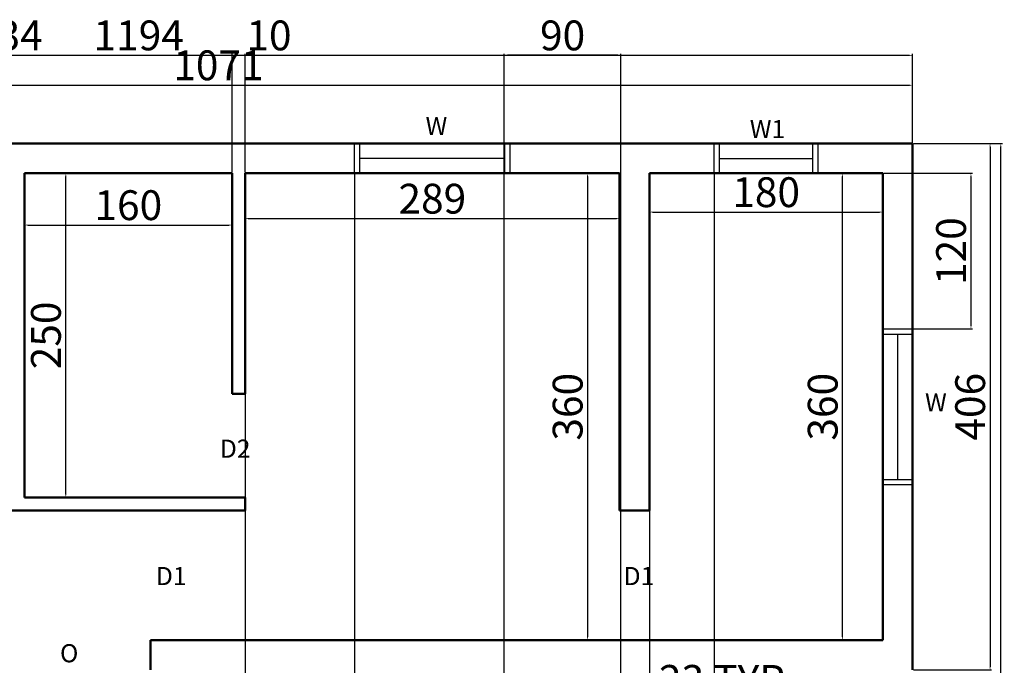
# Model space of a CAD drawing. Units: centimetres. Extents: x 6294 to 7898, y 3240 to 4730.
# Tile 3 of 3: x 6910 to 7669, y 4232 to 4730. Entities that reach past the tile are written whole.
import ezdxf

# ---------------------------------------------------------------- set-up
doc = ezdxf.new("R2010")
doc.units = ezdxf.units.CM
for name, color, linetype, lineweight in [('A-ANNO-DIMS', 2, 'Continuous', 18), ('A-ANNO-TEXT', 7, 'Continuous', 25), ('A-GLAZ', 4, 'Continuous', 25), ('A-WALL', 7, 'Continuous', 50)]:
    doc.layers.add(name, color=color, linetype=linetype, lineweight=lineweight)
doc.styles.get("Standard").update_dxf_attribs({"font": 'arial.ttf'})
doc.dimstyles.new('ISO-25', dxfattribs={"dimtxt": 23, "dimasz": 2.5, "dimexe": 1.25, "dimexo": 0.625, "dimtad": 1, "dimtxsty": 'Standard', "dimcen": 2.5, "dimadec": 0, "dimazin": 0, "dimtfac": 1, "dimtmove": 0, "dimatfit": 3, "dimfxl": 1, "dimarcsym": 0})

# ---------------------------------------------------------------- blocks, each defined once
blk = doc.blocks.new('*D4')
at = {"layer": 'A-ANNO-DIMS', "color": 0, "lineweight": -2, "transparency": 16777216}
for p, q in [((6914.36, 4611.85), (6946.76, 4611.85)), ((6945.51, 4364.35), (6945.51, 4609.35)), ((6914.36, 4361.85), (6946.76, 4361.85))]:
    blk.add_line(p, q, dxfattribs=at)
at = {"layer": 'A-ANNO-DIMS', "color": 0, "transparency": 16777216}
for points in [[(6945.09, 4609.35), (6945.93, 4609.35), (6945.51, 4611.85)], [(6945.09, 4364.35), (6945.93, 4364.35), (6945.51, 4361.85)]]:
    blk.add_solid(points, dxfattribs=at)
at = {"layer": 'Defpoints', "color": 0, "transparency": 16777216}
for p in [(6913.73, 4611.85), (6945.51, 4611.85), (6913.73, 4361.85)]:
    blk.add_point(p, dxfattribs=at)
at = {"layer": 'A-ANNO-DIMS', "color": 0, "transparency": 16777216, "insert": (6933.14, 4486.85), "char_height": 23, "attachment_point": 5, "rotation": 90}
blk.add_mtext('250', dxfattribs=at)
blk = doc.blocks.new('*D5')
at = {"layer": 'A-ANNO-DIMS', "color": 0, "lineweight": -2, "transparency": 16777216}
for p, q in [((6913.73, 4611.22), (6913.73, 4570.69)), ((7073.73, 4611.22), (7073.73, 4570.69)), ((6916.23, 4571.94), (7071.23, 4571.94))]:
    blk.add_line(p, q, dxfattribs=at)
at = {"layer": 'A-ANNO-DIMS', "color": 0, "transparency": 16777216}
for points in [[(6916.23, 4572.35), (6916.23, 4571.52), (6913.73, 4571.94)], [(7071.23, 4572.35), (7071.23, 4571.52), (7073.73, 4571.94)]]:
    blk.add_solid(points, dxfattribs=at)
at = {"layer": 'Defpoints', "color": 0, "transparency": 16777216}
for p in [(6913.73, 4611.85), (7073.73, 4611.85), (7073.73, 4571.94)]:
    blk.add_point(p, dxfattribs=at)
at = {"layer": 'A-ANNO-DIMS', "color": 0, "transparency": 16777216, "insert": (6993.73, 4584.3), "char_height": 23, "attachment_point": 5}
blk.add_mtext('160', dxfattribs=at)
blk = doc.blocks.new('*D6')
at = {"layer": 'A-ANNO-DIMS', "color": 0, "lineweight": -2, "transparency": 16777216}
for p, q in [((7083.73, 4611.22), (7083.73, 4575.69)), ((7372.73, 4611.22), (7372.73, 4575.69)), ((7086.23, 4576.94), (7370.23, 4576.94))]:
    blk.add_line(p, q, dxfattribs=at)
at = {"layer": 'A-ANNO-DIMS', "color": 0, "transparency": 16777216}
for points in [[(7086.23, 4577.36), (7086.23, 4576.52), (7083.73, 4576.94)], [(7370.23, 4577.36), (7370.23, 4576.52), (7372.73, 4576.94)]]:
    blk.add_solid(points, dxfattribs=at)
at = {"layer": 'Defpoints', "color": 0, "transparency": 16777216}
for p in [(7083.73, 4611.85), (7372.73, 4611.85), (7372.73, 4576.94)]:
    blk.add_point(p, dxfattribs=at)
at = {"layer": 'A-ANNO-DIMS', "color": 0, "transparency": 16777216, "insert": (7228.23, 4589.31), "char_height": 23, "attachment_point": 5}
blk.add_mtext('289', dxfattribs=at)
blk = doc.blocks.new('*D7')
at = {"layer": 'A-ANNO-DIMS', "color": 0, "lineweight": -2, "transparency": 16777216}
for p, q in [((7395.73, 4611.22), (7395.73, 4580.7)), ((7575.73, 4611.22), (7575.73, 4580.7)), ((7398.23, 4581.95), (7573.23, 4581.95))]:
    blk.add_line(p, q, dxfattribs=at)
at = {"layer": 'A-ANNO-DIMS', "color": 0, "transparency": 16777216}
for points in [[(7398.23, 4582.36), (7398.23, 4581.53), (7395.73, 4581.95)], [(7573.23, 4582.36), (7573.23, 4581.53), (7575.73, 4581.95)]]:
    blk.add_solid(points, dxfattribs=at)
at = {"layer": 'Defpoints', "color": 0, "transparency": 16777216}
for p in [(7395.73, 4611.85), (7575.73, 4611.85), (7575.73, 4581.95)]:
    blk.add_point(p, dxfattribs=at)
at = {"layer": 'A-ANNO-DIMS', "color": 0, "transparency": 16777216, "insert": (7485.73, 4594.32), "char_height": 23, "attachment_point": 5}
blk.add_mtext('180', dxfattribs=at)
blk = doc.blocks.new('*D8')
at = {"layer": 'A-ANNO-DIMS', "color": 0, "lineweight": -2, "transparency": 16777216}
for p, q in [((7575.11, 4611.85), (7543.48, 4611.85)), ((7544.73, 4254.35), (7544.73, 4609.35)), ((7575.11, 4251.85), (7543.48, 4251.85))]:
    blk.add_line(p, q, dxfattribs=at)
at = {"layer": 'A-ANNO-DIMS', "color": 0, "transparency": 16777216}
for points in [[(7544.32, 4609.35), (7545.15, 4609.35), (7544.73, 4611.85)], [(7544.32, 4254.35), (7545.15, 4254.35), (7544.73, 4251.85)]]:
    blk.add_solid(points, dxfattribs=at)
at = {"layer": 'Defpoints', "color": 0, "transparency": 16777216}
for p in [(7544.73, 4611.85), (7575.73, 4611.85), (7575.73, 4251.85)]:
    blk.add_point(p, dxfattribs=at)
at = {"layer": 'A-ANNO-DIMS', "color": 0, "transparency": 16777216, "insert": (7532.36, 4431.85), "char_height": 23, "attachment_point": 5, "rotation": 90}
blk.add_mtext('360', dxfattribs=at)
blk = doc.blocks.new('*D9')
at = {"layer": 'A-ANNO-DIMS', "color": 0, "lineweight": -2, "transparency": 16777216}
for p, q in [((7372.11, 4611.85), (7346.72, 4611.85)), ((7347.97, 4609.35), (7347.97, 4254.35)), ((7372.11, 4251.85), (7346.72, 4251.85))]:
    blk.add_line(p, q, dxfattribs=at)
at = {"layer": 'A-ANNO-DIMS', "color": 0, "transparency": 16777216}
for points in [[(7347.55, 4609.35), (7348.39, 4609.35), (7347.97, 4611.85)], [(7347.55, 4254.35), (7348.39, 4254.35), (7347.97, 4251.85)]]:
    blk.add_solid(points, dxfattribs=at)
at = {"layer": 'Defpoints', "color": 0, "transparency": 16777216}
for p in [(7372.73, 4611.85), (7347.97, 4251.85), (7372.73, 4251.85)]:
    blk.add_point(p, dxfattribs=at)
at = {"layer": 'A-ANNO-DIMS', "color": 0, "transparency": 16777216, "insert": (7335.59, 4431.85), "char_height": 23, "attachment_point": 5, "rotation": 90}
blk.add_mtext('360', dxfattribs=at)
blk = doc.blocks.new('*D23')
at = {"layer": 'A-ANNO-DIMS', "color": 0, "lineweight": -2, "transparency": 16777216}
for p, q in [((6527.73, 4635.47), (6527.73, 4681.05)), ((6530.23, 4679.8), (7596.23, 4679.8)), ((7598.73, 4635.47), (7598.73, 4681.05))]:
    blk.add_line(p, q, dxfattribs=at)
at = {"layer": 'A-ANNO-DIMS', "color": 0, "transparency": 16777216}
for points in [[(6530.23, 4680.22), (6530.23, 4679.38), (6527.73, 4679.8)], [(7596.23, 4680.22), (7596.23, 4679.38), (7598.73, 4679.8)]]:
    blk.add_solid(points, dxfattribs=at)
at = {"layer": 'Defpoints', "color": 0, "transparency": 16777216}
for p in [(7598.73, 4679.8), (6527.73, 4634.85), (7598.73, 4634.85)]:
    blk.add_point(p, dxfattribs=at)
at = {"layer": 'A-ANNO-DIMS', "color": 0, "transparency": 16777216, "insert": (7063.23, 4692.17), "char_height": 23, "attachment_point": 5}
blk.add_mtext('1071', dxfattribs=at)
blk = doc.blocks.new('*D24')
at = {"layer": 'A-ANNO-DIMS', "color": 0, "lineweight": -2, "transparency": 16777216}
for p, q in [((7599.36, 4634.85), (7659.7, 4634.85)), ((7658.45, 4632.35), (7658.45, 4231.35)), ((7599.36, 4228.85), (7659.7, 4228.85))]:
    blk.add_line(p, q, dxfattribs=at)
at = {"layer": 'A-ANNO-DIMS', "color": 0, "transparency": 16777216}
for points in [[(7658.04, 4632.35), (7658.87, 4632.35), (7658.45, 4634.85)], [(7658.04, 4231.35), (7658.87, 4231.35), (7658.45, 4228.85)]]:
    blk.add_solid(points, dxfattribs=at)
at = {"layer": 'Defpoints', "color": 0, "transparency": 16777216}
for p in [(7598.73, 4634.85), (7598.73, 4228.85), (7658.45, 4228.85)]:
    blk.add_point(p, dxfattribs=at)
at = {"layer": 'A-ANNO-DIMS', "color": 0, "transparency": 16777216, "insert": (7646.08, 4431.85), "char_height": 23, "attachment_point": 5, "rotation": 90}
blk.add_mtext('406', dxfattribs=at)
blk = doc.blocks.new('WIN-W-120CM')
for p, q in [((0, 23), (0, 0)), ((4, 23), (4, 0)), ((116, 23), (116, 0)), ((120, 23), (120, 0)), ((4, 11.5), (116, 11.5))]:
    blk.add_line(p, q)
blk = doc.blocks.new('FRAME-W1-V-80CM')
for p, q in [((0, 0), (0, 23)), ((4, 0), (4, 23)), ((76, 0), (76, 23)), ((80, 0), (80, 23)), ((4, 11.5), (76, 11.5))]:
    blk.add_line(p, q)
blk = doc.blocks.new('*D35')
at = {"layer": 'A-ANNO-DIMS', "color": 0, "lineweight": -2, "transparency": 16777216}
for p, q in [((7373.73, 4194.47), (7373.73, 4207.1)), ((7376.23, 4205.85), (7394.23, 4205.85)), ((7396.73, 4194.47), (7396.73, 4207.1)), ((7396.73, 4205.85), (7512.83, 4205.85))]:
    blk.add_line(p, q, dxfattribs=at)
at = {"layer": 'A-ANNO-DIMS', "color": 0, "transparency": 16777216}
for points in [[(7376.23, 4206.26), (7376.23, 4205.43), (7373.73, 4205.85)], [(7394.23, 4206.26), (7394.23, 4205.43), (7396.73, 4205.85)]]:
    blk.add_solid(points, dxfattribs=at)
at = {"layer": 'Defpoints', "color": 0, "transparency": 16777216}
for p in [(7396.73, 4205.85), (7373.73, 4193.85), (7396.73, 4193.85)]:
    blk.add_point(p, dxfattribs=at)
at = {"layer": 'A-ANNO-DIMS', "color": 0, "transparency": 16777216, "insert": (7456.03, 4218.22), "char_height": 23, "attachment_point": 5}
blk.add_mtext('23 TYP.', dxfattribs=at)
blk = doc.blocks.new('*D38')
at = {"layer": 'A-ANNO-DIMS', "color": 0, "lineweight": -2, "transparency": 16777216}
for p, q in [((7599.36, 4634.85), (7667.98, 4634.85)), ((7666.73, 3313.35), (7666.73, 4632.35)), ((7397.36, 3310.85), (7667.98, 3310.85))]:
    blk.add_line(p, q, dxfattribs=at)
at = {"layer": 'A-ANNO-DIMS', "color": 0, "transparency": 16777216}
for points in [[(7666.32, 4632.35), (7667.15, 4632.35), (7666.73, 4634.85)], [(7666.32, 3313.35), (7667.15, 3313.35), (7666.73, 3310.85)]]:
    blk.add_solid(points, dxfattribs=at)
at = {"layer": 'Defpoints', "color": 0, "transparency": 16777216}
for p in [(7598.73, 4634.85), (7666.73, 4634.85), (7396.73, 3310.85)]:
    blk.add_point(p, dxfattribs=at)
at = {"layer": 'A-ANNO-DIMS', "color": 0, "transparency": 16777216, "insert": (7654.36, 3972.85), "char_height": 23, "attachment_point": 5, "rotation": 90}
blk.add_mtext('1324', dxfattribs=at)
blk = doc.blocks.new('*D39')
at = {"layer": 'A-ANNO-DIMS', "color": 0, "lineweight": -2, "transparency": 16777216}
for p, q in [((6404.73, 4129.47), (6404.73, 4704.1)), ((6407.23, 4702.85), (7596.23, 4702.85)), ((7598.73, 4635.47), (7598.73, 4704.1))]:
    blk.add_line(p, q, dxfattribs=at)
at = {"layer": 'A-ANNO-DIMS', "color": 0, "transparency": 16777216}
for points in [[(6407.23, 4703.26), (6407.23, 4702.43), (6404.73, 4702.85)], [(7596.23, 4703.26), (7596.23, 4702.43), (7598.73, 4702.85)]]:
    blk.add_solid(points, dxfattribs=at)
at = {"layer": 'Defpoints', "color": 0, "transparency": 16777216}
for p in [(7598.73, 4702.85), (7598.73, 4634.85), (6404.73, 4128.85)]:
    blk.add_point(p, dxfattribs=at)
at = {"layer": 'A-ANNO-DIMS', "color": 0, "transparency": 16777216, "insert": (7001.73, 4715.22), "char_height": 23, "attachment_point": 5}
blk.add_mtext('1194', dxfattribs=at)
blk = doc.blocks.new('*D40')
at = {"layer": 'A-ANNO-DIMS', "color": 0, "lineweight": -2, "transparency": 16777216}
for p, q in [((6856.73, 4029.47), (6856.73, 4704.1)), ((6859.23, 4702.85), (6888.23, 4702.85)), ((6890.73, 4029.47), (6890.73, 4704.1)), ((6890.73, 4702.85), (6927.32, 4702.85))]:
    blk.add_line(p, q, dxfattribs=at)
at = {"layer": 'A-ANNO-DIMS', "color": 0, "transparency": 16777216}
for points in [[(6859.23, 4703.26), (6859.23, 4702.43), (6856.73, 4702.85)], [(6888.23, 4703.26), (6888.23, 4702.43), (6890.73, 4702.85)]]:
    blk.add_solid(points, dxfattribs=at)
at = {"layer": 'Defpoints', "color": 0, "transparency": 16777216}
for p in [(6890.73, 4702.85), (6856.73, 4028.85), (6890.73, 4028.85)]:
    blk.add_point(p, dxfattribs=at)
at = {"layer": 'A-ANNO-DIMS', "color": 0, "transparency": 16777216, "insert": (6910.28, 4715.22), "char_height": 23, "attachment_point": 5}
blk.add_mtext('34', dxfattribs=at)
blk = doc.blocks.new('*D46')
at = {"layer": 'A-ANNO-DIMS', "color": 0, "lineweight": -2, "transparency": 16777216}
for p, q in [((7083.73, 4611.22), (7083.73, 3241.6)), ((7168.23, 4611.22), (7168.23, 3241.6)), ((7086.23, 3242.85), (7165.73, 3242.85))]:
    blk.add_line(p, q, dxfattribs=at)
at = {"layer": 'A-ANNO-DIMS', "color": 0, "transparency": 16777216}
for points in [[(7086.23, 3243.26), (7086.23, 3242.43), (7083.73, 3242.85)], [(7165.73, 3243.26), (7165.73, 3242.43), (7168.23, 3242.85)]]:
    blk.add_solid(points, dxfattribs=at)
at = {"layer": 'Defpoints', "color": 0, "transparency": 16777216}
for p in [(7083.73, 4611.85), (7168.23, 4611.85), (7168.23, 3242.85)]:
    blk.add_point(p, dxfattribs=at)
at = {"layer": 'A-ANNO-DIMS', "color": 0, "transparency": 16777216, "insert": (7125.98, 3255.22), "char_height": 23, "attachment_point": 5}
blk.add_mtext('84.5', dxfattribs=at)
blk = doc.blocks.new('*D47')
at = {"layer": 'A-ANNO-DIMS', "color": 0, "lineweight": -2, "transparency": 16777216}
for p, q in [((7395.73, 4611.22), (7395.73, 3241.6)), ((7445.73, 4611.22), (7445.73, 3241.6)), ((7398.23, 3242.85), (7443.23, 3242.85))]:
    blk.add_line(p, q, dxfattribs=at)
at = {"layer": 'A-ANNO-DIMS', "color": 0, "transparency": 16777216}
for points in [[(7398.23, 3243.26), (7398.23, 3242.43), (7395.73, 3242.85)], [(7443.23, 3243.26), (7443.23, 3242.43), (7445.73, 3242.85)]]:
    blk.add_solid(points, dxfattribs=at)
at = {"layer": 'Defpoints', "color": 0, "transparency": 16777216}
for p in [(7395.73, 4611.85), (7445.73, 4611.85), (7445.73, 3242.85)]:
    blk.add_point(p, dxfattribs=at)
at = {"layer": 'A-ANNO-DIMS', "color": 0, "transparency": 16777216, "insert": (7420.73, 3255.22), "char_height": 23, "attachment_point": 5}
blk.add_mtext('50', dxfattribs=at)
blk = doc.blocks.new('*D50')
at = {"layer": 'A-ANNO-DIMS', "color": 0, "lineweight": -2, "transparency": 16777216}
for p, q in [((7283.73, 3717.47), (7283.73, 4704.1)), ((7371.23, 4702.85), (7286.23, 4702.85)), ((7373.73, 3717.47), (7373.73, 4704.1))]:
    blk.add_line(p, q, dxfattribs=at)
at = {"layer": 'A-ANNO-DIMS', "color": 0, "transparency": 16777216}
for points in [[(7286.23, 4703.26), (7286.23, 4702.43), (7283.73, 4702.85)], [(7371.23, 4703.26), (7371.23, 4702.43), (7373.73, 4702.85)]]:
    blk.add_solid(points, dxfattribs=at)
at = {"layer": 'Defpoints', "color": 0, "transparency": 16777216}
for p in [(7283.73, 4702.85), (7283.73, 3716.85), (7373.73, 3716.85)]:
    blk.add_point(p, dxfattribs=at)
at = {"layer": 'A-ANNO-DIMS', "color": 0, "transparency": 16777216, "insert": (7328.73, 4715.22), "char_height": 23, "attachment_point": 5}
blk.add_mtext('90', dxfattribs=at)
blk = doc.blocks.new('*D51')
at = {"layer": 'A-ANNO-DIMS', "color": 0, "lineweight": -2, "transparency": 16777216}
for p, q in [((7073.73, 4612.47), (7073.73, 4704.1)), ((7076.23, 4702.85), (7081.23, 4702.85)), ((7083.73, 4612.47), (7083.73, 4704.1)), ((7083.73, 4702.85), (7118.19, 4702.85))]:
    blk.add_line(p, q, dxfattribs=at)
at = {"layer": 'A-ANNO-DIMS', "color": 0, "transparency": 16777216}
for points in [[(7076.23, 4703.26), (7076.23, 4702.43), (7073.73, 4702.85)], [(7081.23, 4703.26), (7081.23, 4702.43), (7083.73, 4702.85)]]:
    blk.add_solid(points, dxfattribs=at)
at = {"layer": 'Defpoints', "color": 0, "transparency": 16777216}
for p in [(7083.73, 4702.85), (7073.73, 4611.85), (7083.73, 4611.85)]:
    blk.add_point(p, dxfattribs=at)
at = {"layer": 'A-ANNO-DIMS', "color": 0, "transparency": 16777216, "insert": (7102.21, 4715.22), "char_height": 23, "attachment_point": 5}
blk.add_mtext('10', dxfattribs=at)
blk = doc.blocks.new('*D53')
at = {"layer": 'A-ANNO-DIMS', "color": 0, "lineweight": -2, "transparency": 16777216}
for p, q in [((7576.36, 4611.85), (7644.98, 4611.85)), ((7643.73, 4609.35), (7643.73, 4494.35)), ((7576.36, 4491.85), (7644.98, 4491.85))]:
    blk.add_line(p, q, dxfattribs=at)
at = {"layer": 'A-ANNO-DIMS', "color": 0, "transparency": 16777216}
for points in [[(7643.32, 4609.35), (7644.15, 4609.35), (7643.73, 4611.85)], [(7643.32, 4494.35), (7644.15, 4494.35), (7643.73, 4491.85)]]:
    blk.add_solid(points, dxfattribs=at)
at = {"layer": 'Defpoints', "color": 0, "transparency": 16777216}
for p in [(7575.73, 4611.85), (7575.73, 4491.85), (7643.73, 4491.85)]:
    blk.add_point(p, dxfattribs=at)
at = {"layer": 'A-ANNO-DIMS', "color": 0, "transparency": 16777216, "insert": (7631.37, 4551.85), "char_height": 23, "attachment_point": 5, "rotation": 90}
blk.add_mtext('120', dxfattribs=at)

msp = doc.modelspace()

# ---------------------------------------------------------------- linework, layer by layer
at = {"layer": 'A-WALL'}
for p, q in [((7598.735, 4634.848), (6527.735, 4634.848)), ((7598.735, 4634.848), (7598.735, 4228.848)), ((6913.735, 4611.848), (6913.735, 4361.848)), ((7073.735, 4611.848), (6913.735, 4611.848)), ((7073.735, 4611.848), (7073.735, 4441.848)), ((7083.735, 4611.848), (7083.735, 4441.848)), ((7372.735, 4611.848), (7083.735, 4611.848)), ((7372.735, 4611.848), (7372.735, 4351.848)), ((7575.735, 4611.848), (7395.735, 4611.848)), ((7395.735, 4611.848), (7395.735, 4351.848)), ((7575.735, 4611.848), (7575.735, 4251.848)), ((7083.735, 4441.848), (7073.735, 4441.848)), ((7083.735, 4361.848), (6913.735, 4361.848)), ((7083.735, 4361.848), (7083.735, 4351.848)), ((7083.735, 4351.848), (6890.735, 4351.848)), ((7395.735, 4351.848), (7372.735, 4351.848)), ((7575.735, 4251.848), (7010.735, 4251.848)), ((7010.735, 4251.848), (7010.735, 4228.848))]:
    msp.add_line(p, q, dxfattribs=at)

# ---------------------------------------------------------------- block references
at = {"layer": 'A-GLAZ'}
for p, rotation in [((7288.235, 4634.848), 180), ((7598.735, 4371.848), 90.00000000000152)]:
    msp.add_blockref('WIN-W-120CM', p, dxfattribs=dict(at, rotation=rotation))
msp.add_blockref('FRAME-W1-V-80CM', (7445.735, 4611.848), dxfattribs=at)

# ---------------------------------------------------------------- texts
at = {"layer": 'A-ANNO-TEXT'}
for s, height, p in [('W', 13.978, (7223.014, 4641.332)), ('W1', 13.9778, (7473.12, 4638.976)), ('W', 13.978, (7608.31, 4428.179)), ('D2', 13.9778, (7064.29, 4392.516)), ('D1', 13.9778, (7014.978, 4294.279)), ('D1', 13.9778, (7375.778, 4294.279)), ('O ', 13.9778, (6941.027, 4234.761))]:
    msp.add_text(s, height=height, dxfattribs=at).set_placement(p)

# ---------------------------------------------------------------- dimensions: what is measured, and where the dimension line sits
at = {"layer": 'A-ANNO-DIMS'}
for base, p1, p2, override, picture, middle in [((7598.735, 4702.848), (6404.735, 4128.848), (7598.735, 4634.848), {"dimdec": 0, "dimlfac": 1, "dimrnd": 0, "dimzin": 0, "dimdsep": 46, "dimlunit": 2}, '*D39', (7001.735, 4715.216)), ((6890.735, 4702.848), (6856.735, 4028.848), (6890.735, 4028.848), {"dimdec": 0, "dimlfac": 1, "dimrnd": 0, "dimzin": 0, "dimdsep": 46, "dimlunit": 2}, '*D40', (6910.278, 4715.224)), ((7083.735, 4702.848), (7073.735, 4611.848), (7083.735, 4611.848), {"dimdec": 0, "dimlfac": 1, "dimrnd": 0, "dimzin": 0, "dimdsep": 46, "dimlunit": 2}, '*D51', (7102.211, 4715.216)), ((7283.735, 4702.848), (7373.735, 3716.848), (7283.735, 3716.848), {"dimdec": 0, "dimlfac": 1, "dimrnd": 0, "dimzin": 0, "dimdsep": 46, "dimlunit": 2}, '*D50', (7328.735, 4715.216)), ((7598.735, 4679.801), (6527.735, 4634.848), (7598.735, 4634.848), {"dimclrd": 0, "dimclre": 0, "dimclrt": 0}, '*D23', (7063.235, 4692.17)), ((7073.735, 4571.936), (6913.735, 4611.848), (7073.735, 4611.848), {"dimclrd": 0, "dimclre": 0, "dimclrt": 0}, '*D5', (6993.735, 4584.304)), ((7372.735, 4576.941), (7083.735, 4611.848), (7372.735, 4611.848), {"dimclrd": 0, "dimclre": 0, "dimclrt": 0}, '*D6', (7228.235, 4589.309)), ((7168.235, 3242.848), (7083.735, 4611.848), (7168.235, 4611.848), {"dimdec": 1, "dimlfac": 1, "dimrnd": 0, "dimzin": 0, "dimdsep": 46, "dimlunit": 2}, '*D46', (7125.985, 3255.216)), ((7575.735, 4581.948), (7395.735, 4611.848), (7575.735, 4611.848), {"dimclrd": 0, "dimclre": 0, "dimclrt": 0}, '*D7', (7485.735, 4594.316)), ((7445.735, 3242.848), (7395.735, 4611.848), (7445.735, 4611.848), {"dimdec": 0, "dimlfac": 1, "dimrnd": 0, "dimzin": 0, "dimdsep": 46, "dimlunit": 2}, '*D47', (7420.735, 3255.216))]:
    dim = msp.add_linear_dim(base=base, p1=p1, p2=p2, dimstyle='ISO-25', override=override, dxfattribs=at)
    dim.commit()
    dim.dimension.update_dxf_attribs({"geometry": picture, "text_midpoint": middle})
for base, p1, p2, angle, override, picture, middle in [((7666.735, 4634.848), (7396.735, 3310.848), (7598.735, 4634.848), 90, {"dimdec": 0, "dimlfac": 1, "dimrnd": 0, "dimzin": 0, "dimdsep": 46, "dimlunit": 2}, '*D38', (7654.359, 3972.848)), ((7658.452, 4228.848), (7598.735, 4634.848), (7598.735, 4228.848), 90, {"dimclrd": 0, "dimclre": 0, "dimclrt": 0}, '*D24', (7646.084, 4431.848)), ((6945.509, 4611.848), (6913.735, 4361.848), (6913.735, 4611.848), 270, {"dimclrd": 0, "dimclre": 0, "dimclrt": 0}, '*D4', (6933.14, 4486.848)), ((7347.971, 4251.848), (7372.735, 4611.848), (7372.735, 4251.848), 90, {"dimclrd": 0, "dimclre": 0, "dimclrt": 0}, '*D9', (7335.595, 4431.848)), ((7544.734, 4611.848), (7575.735, 4251.848), (7575.735, 4611.848), 270, {"dimclrd": 0, "dimclre": 0, "dimclrt": 0}, '*D8', (7532.358, 4431.848)), ((7643.735, 4491.848), (7575.735, 4611.848), (7575.735, 4491.848), 270, {"dimdec": 0, "dimlfac": 1, "dimrnd": 0, "dimzin": 0, "dimdsep": 46, "dimlunit": 2}, '*D53', (7631.366, 4551.848))]:
    dim = msp.add_linear_dim(base=base, p1=p1, p2=p2, angle=angle, dimstyle='ISO-25', override=override, dxfattribs=at)
    dim.commit()
    dim.dimension.update_dxf_attribs({"geometry": picture, "text_midpoint": middle})
dim = msp.add_linear_dim(base=(7396.735, 4205.848), p1=(7373.735, 4193.848), p2=(7396.735, 4193.848), text='<> TYP.', dimstyle='ISO-25', override={"dimdec": 0, "dimlfac": 1, "dimrnd": 0, "dimzin": 0, "dimdsep": 46, "dimlunit": 2}, dxfattribs=at)
dim.commit()
dim.dimension.update_dxf_attribs({"geometry": '*D35', "text_midpoint": (7456.034, 4218.224)})

doc.saveas('drawing.dxf')
